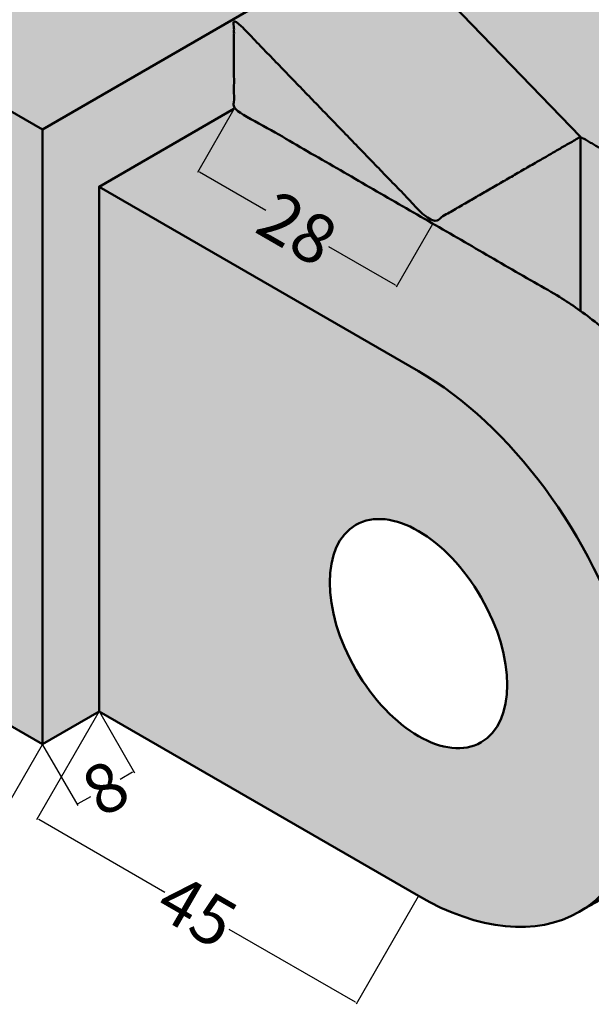
# Model space of a CAD drawing. Units: millimetres. Extents: x -24 to 183, y 0 to 191.
# Tile 1 of 1: x 51 to 120.7, y -0.5 to 119.6. Entities that reach past the tile are written whole.
import ezdxf

# ---------------------------------------------------------------- set-up
doc = ezdxf.new("R2010")
doc.units = ezdxf.units.MM
doc.header["$MEASUREMENT"] = 0
for name, color, linetype, lineweight in [('M-DIMS', 2, 'Continuous', 25), ('M-HATC', 7, 'Continuous', 18), ('M-OUTL', 7, 'Continuous', 50)]:
    doc.layers.add(name, color=color, linetype=linetype, lineweight=lineweight)
doc.styles.get("Standard").update_dxf_attribs({"font": 'arial.ttf'})
doc.dimstyles.get("Standard").update_dxf_attribs({"dimtxt": 6, "dimasz": 0.18, "dimexe": 0.18, "dimexo": 0.0625, "dimgap": 0.09, "dimtad": 0, "dimtoh": 1, "dimdec": 0, "dimzin": 0, "dimdsep": 46, "dimtxsty": 'Standard', "dimcen": 0.09, "dimadec": 0, "dimazin": 0, "dimtfac": 1, "dimtdec": 0, "dimtofl": 0, "dimtmove": 0, "dimatfit": 3, "dimfxl": 1, "dimtolj": 1, "dimtzin": 0, "dimarcsym": 0})

# ---------------------------------------------------------------- blocks, each defined once
blk = doc.blocks.new('*D2')
at = {"layer": 'Defpoints', "color": 0, "transparency": 16777216}
for p in [(77.13283570151157, 108.711638219327), (101.3815470074758, 94.71163821932711), (96.99877424901707, 87.1204531236477)]:
    blk.add_point(p, dxfattribs=at)
at = {"layer": 'M-DIMS', "color": 0, "lineweight": -2, "transparency": 16777216}
for p, q in [((77.10158570151157, 108.6575116315905), (72.6600629430528, 100.9645685509665)), ((72.905947515734, 101.0304531236477), (81.02518969457847, 96.34280646607608)), ((101.3502970074758, 94.65751163159058), (96.90877424901707, 86.9645685509665)), ((96.84288967633589, 87.2104531236477), (88.7236474974914, 91.89809978121934))]:
    blk.add_line(p, q, dxfattribs=at)
at = {"layer": 'M-DIMS', "color": 0, "transparency": 16777216}
for points in [[(72.920947515734, 101.0564338857612), (72.890947515734, 101.0044723615341), (72.7500629430528, 101.1204531236477)], [(96.85788967633587, 87.23643388576124), (96.82788967633587, 87.18447236153418), (96.99877424901707, 87.1204531236477)]]:
    blk.add_solid(points, dxfattribs=at)
at = {"layer": 'M-DIMS', "color": 0, "transparency": 16777216, "insert": (84.87441859603494, 94.1204531236477), "char_height": 6, "attachment_point": 5, "rotation": 330}
blk.add_mtext('\\A1;28', dxfattribs=at)
blk = doc.blocks.new('*D7')
at = {"layer": 'Defpoints', "color": 0, "transparency": 16777216}
for p in [(-0.8094506390879097, 62.71163821932709), (53.75014979933173, 31.2116382193271), (48.99750972183936, 22.97982413502221)]:
    blk.add_point(p, dxfattribs=at)
at = {"layer": 'M-DIMS', "color": 0, "lineweight": -2, "transparency": 16777216}
for p, q in [((-0.8407006390879097, 62.65751163159055), (-5.652090716580296, 54.32393956234097)), ((-5.406206143899098, 54.38982413502217), (17.90392502424746, 40.93171363024729)), ((48.84162514915816, 23.06982413502221), (25.53149398101159, 36.5279346397971)), ((53.71889979933173, 31.15751163159057), (48.90750972183936, 22.82393956234101))]:
    blk.add_line(p, q, dxfattribs=at)
at = {"layer": 'M-DIMS', "color": 0, "transparency": 16777216}
for points in [[(-5.391206143899097, 54.41580489713571), (-5.421206143899098, 54.36384337290864), (-5.562090716580296, 54.47982413502217)], [(48.85662514915816, 23.09580489713574), (48.82662514915816, 23.04384337290867), (48.99750972183936, 22.97982413502221)]]:
    blk.add_solid(points, dxfattribs=at)
at = {"layer": 'M-DIMS', "color": 0, "transparency": 16777216, "insert": (21.71770950262953, 38.72982413502219), "char_height": 6, "attachment_point": 5, "rotation": 330}
blk.add_mtext('\\A1;63', dxfattribs=at)
blk = doc.blocks.new('*D8')
at = {"layer": 'Defpoints', "color": 0, "transparency": 16777216}
for p in [(60.67835302960723, 35.21163821932709), (53.75014979933173, 31.2116382193271), (64.90447024958932, 27.89178847557638)]:
    blk.add_point(p, dxfattribs=at)
at = {"layer": 'M-DIMS', "color": 0, "lineweight": -2, "transparency": 16777216}
for p, q in [((60.70960302960724, 35.15751163159056), (64.99447024958933, 27.73590390289518)), ((53.78139979933172, 31.15751163159057), (58.06626701931381, 23.73590390289518)), ((64.74858567690812, 27.80178847557637), (63.23027655528555, 26.92519229549452)), ((58.13215159199502, 23.98178847557637), (59.65046071361759, 24.85838465565823))]:
    blk.add_line(p, q, dxfattribs=at)
at = {"layer": 'M-DIMS', "color": 0, "transparency": 16777216}
for points in [[(64.73358567690812, 27.8277692376899), (64.76358567690812, 27.77580771346284), (64.90447024958932, 27.89178847557638)], [(58.11715159199501, 24.00776923768991), (58.14715159199502, 23.95580771346284), (57.97626701931381, 23.89178847557637)]]:
    blk.add_solid(points, dxfattribs=at)
at = {"layer": 'M-DIMS', "color": 0, "transparency": 16777216, "insert": (61.44036863445157, 25.89178847557637), "char_height": 6, "attachment_point": 5, "rotation": 30.000000000000025}
blk.add_mtext('\\A1;8', dxfattribs=at)
blk = doc.blocks.new('*D9')
at = {"layer": 'Defpoints', "color": 0, "transparency": 16777216}
for p in [(60.67835302960723, 35.2116382193271), (99.64949619990699, 12.7116382193271), (92.11221586893467, -0.3433142648065512)]:
    blk.add_point(p, dxfattribs=at)
at = {"layer": 'M-DIMS', "color": 0, "lineweight": -2, "transparency": 16777216}
for p, q in [((60.64710302960723, 35.15751163159057), (53.0510726986349, 22.00080116251224)), ((53.2969572713161, 22.06668573519343), (68.70298209387207, 13.1720131567487)), ((99.618246199907, 12.65751163159057), (92.02221586893467, -0.4991988374877466)), ((91.95633129625347, -0.2533142648065478), (76.55030647369747, 8.6413583136382))]:
    blk.add_line(p, q, dxfattribs=at)
at = {"layer": 'M-DIMS', "color": 0, "transparency": 16777216}
for points in [[(53.31195727131611, 22.09266649730697), (53.2819572713161, 22.0407049730799), (53.1410726986349, 22.15668573519343)], [(91.97133129625345, -0.2273335026930141), (91.94133129625345, -0.2792950269200816), (92.11221586893467, -0.3433142648065512)]]:
    blk.add_solid(points, dxfattribs=at)
at = {"layer": 'M-DIMS', "color": 0, "transparency": 16777216, "insert": (72.62664428378477, 10.90668573519344), "char_height": 6, "attachment_point": 5, "rotation": 330}
blk.add_mtext('\\A1;45', dxfattribs=at)

msp = doc.modelspace()

# ---------------------------------------------------------------- hatches: boundary and pattern name
at = {"layer": 'M-HATC'}
h = msp.add_hatch(color=256, dxfattribs=at)
h.set_gradient(color1=(244, 238, 81), color2=(244, 238, 81), tint=1)
h.paths.add_polyline_path([(64.14245464474502, 175.211638219327), (-0.8094506390879131, 137.7116382193271), (53.75014979933173, 106.2116382193271), (118.7020550831646, 143.7116382193271)])
edge = h.paths.add_edge_path()
edge.add_line((95.31936918098478, 130.2116382193271), (77.13283570151161, 119.7116382193271))
edge.add_spline(control_points=[(77.13283570151158, 119.7116382193271), (89.17924906810929, 107.2566382193724), (101.2256624347508, 94.80163821937239)], knot_values=[5.356194490192345, 5.356194490192345, 5.356194490192345, 6.356194490188707, 6.356194490192345, 6.356194490192345], weights=[1, 1, 1], degree=2, periodic=0)
edge.add_spline(control_points=[(101.2256624347947, 94.80163821932707), (110.3189291745312, 100.051638219327), (119.4121959142679, 105.301638219327)], knot_values=[6.356194490188707, 6.356194490192345, 6.356194490192345, 7.356194490192345, 7.356194490192345, 7.356194490192345], weights=[1, 1, 1], degree=2, periodic=0)
edge.add_line((119.4121959142679, 105.3016382193271), (95.31936918098478, 130.2116382193271))
edge = h.paths.add_edge_path()
edge.add_spline(control_points=[(150.7449950231889, 106.2116382193271), (134.7235250531767, 115.4616382193271), (118.7020550831646, 124.7116382193271)], knot_values=[3.356194490192345, 3.356194490192345, 3.356194490192345, 4.178416712414569, 4.178416712414569, 4.178416712414569], weights=[1, 1, 1], degree=2, periodic=0)
edge.add_spline(control_points=[(118.7020550831646, 124.7116382193271), (115.2379534680269, 126.7116382193271), (111.7738518528891, 128.7116382193271)], knot_values=[4.178416712414569, 4.178416712414569, 4.178416712414569, 4.356194490192345, 4.356194490192345, 4.356194490192345], weights=[1, 1, 1], degree=2, periodic=0)
edge.add_spline(control_points=[(111.7738518528891, 128.7116382193271), (106.960071285434, 125.9324007128871), (102.1462907179789, 123.1531632064471)], knot_values=[4.356194490192345, 4.356194490192345, 4.356194490192345, 5.356194490192345, 5.356194490192345, 5.356194490192345], weights=[1, 1, 1], degree=2, periodic=0)
edge.add_line((102.1462907179789, 123.1531632064471), (119.4121959142679, 105.301638219327))
edge.add_spline(control_points=[(119.4121959142679, 105.301638219327), (126.8513541327762, 101.006638219327), (134.2905123512845, 96.71163821932709)], knot_values=[7.356194490192345, 7.356194490192345, 7.356194490192345, 8.356194490192346, 8.356194490192346, 8.356194490192346], weights=[1, 1, 1], degree=2, periodic=0)
edge.add_spline(control_points=[(134.2905123512845, 96.71163821932709), (158.0953395036126, 82.96791485491796), (161.6862132372617, 53.72180942535438), (165.2770869709107, 24.47570399579081), (142.5556009483879, 29.39608484008592)], knot_values=[8.356194490192346, 8.356194490192346, 8.356194490192346, 9.775566349411587, 9.775566349411587, 11.19493820863083, 11.19493820863083, 11.19493820863083], weights=[1, 0.7585665602715825, 1, 0.7585665602715825, 1], degree=2, periodic=0)
edge.add_spline(control_points=[(153.8864302935499, 30.77051272237281), (162.1136716295021, 35.52051272237281), (170.3409129654543, 40.2705127223728)], knot_values=[0, 0, 0, 1, 1, 1], weights=[1, 1, 1], degree=2, periodic=0)
edge.add_spline(control_points=[(170.3409129654543, 40.2705127223728), (183.4344867248955, 47.83009105704043), (176.3482956693094, 71.67543553482938), (169.2621046137232, 95.5207800126183), (150.7449950231889, 106.2116382193271)], knot_values=[1, 1, 1, 2.178097245096171, 2.178097245096171, 3.356194490192345, 3.356194490192345, 3.356194490192345], weights=[1, 0.831469612302545, 1, 0.831469612302545, 1], degree=2, periodic=0)
edge = h.paths.add_edge_path(flags=17)
edge.add_spline(control_points=[(134.2905123512845, 96.71163821932709), (126.8513541327762, 101.006638219327), (119.4121959142679, 105.301638219327)], knot_values=[7.356194490192345, 7.356194490192345, 7.356194490192345, 8.356194490192346, 8.356194490192346, 8.356194490192346], weights=[1, 1, 1], degree=2, periodic=0)
edge.add_line((119.4121959142679, 105.301638219327), (119.4121959142679, 84.07281383496964))
edge.add_spline(control_points=[(119.4121959142679, 84.07281383496964), (123.0724490086632, 81.4513939238958), (126.4903518736498, 77.88262675949477)], knot_values=[2.966768687208849, 2.966768687208849, 2.966768687208849, 3.231438789490306, 3.231438789490306, 3.231438789490306], weights=[0.9680864183363699, 0.938243390584542, 0.9254123758008628], degree=2, periodic=0)
edge.add_ellipse((134.2905123512845, 64.71163821932709), major_axis=(7.654655446197426, -13.25825214724777), ratio=0.5773502691896262, start_angle=359.3650130620468, end_angle=540.634986937953, ccw=False)
edge.add_spline(control_points=[(141.7968427812057, 51.37100682201758), (145.5119247027769, 38.61436904653682), (142.5556009483879, 29.39608484008592)], knot_values=[1.485548755374229, 1.485548755374229, 1.485548755374229, 2.169061485720957, 2.169061485720957, 2.169061485720957], weights=[0.9974346422091759, 0.9011559533067647, 0.9183363162707197], degree=2, periodic=0)
edge.add_spline(control_points=[(142.5556009483879, 29.39608484008592), (165.2770869709107, 24.47570399579081), (161.6862132372617, 53.72180942535438), (158.0953395036126, 82.96791485491796), (134.2905123512845, 96.71163821932709)], knot_values=[8.356194490192342, 8.356194490192342, 8.356194490192342, 9.775566349411587, 9.775566349411587, 11.19493820863083, 11.19493820863083, 11.19493820863083], weights=[1, 0.7585665602715825, 1, 0.7585665602715825, 1], degree=2, periodic=0)
edge = h.paths.add_edge_path()
edge.add_spline(control_points=[(119.4121959142679, 105.301638219327), (110.3189291745312, 100.051638219327), (101.2256624347947, 94.80163821932707)], knot_values=[6.356194490188707, 6.356194490188707, 6.356194490188707, 7.356194490188707, 7.356194490188707, 7.356194490192345], weights=[1, 1, 1], degree=2, periodic=0)
edge.add_spline(control_points=[(101.2256624347947, 94.80163821932709), (108.664820653303, 90.5066382193271), (116.1039788718113, 86.21163821932711)], knot_values=[3.356194490192346, 3.356194490192346, 3.356194490192346, 3.737972267970123, 3.737972267970123, 3.737972267970123], weights=[1, 1, 1], degree=2, periodic=0)
edge.add_spline(control_points=[(116.1039788718113, 86.21163821932711), (117.7640226821475, 85.25321147856292), (119.4121959142679, 84.07281383496964)], knot_values=[3.231438789490306, 3.231438789490306, 3.231438789490306, 3.356194490192346, 3.356194490192346, 3.356194490192346], weights=[1, 0.9821533182474542, 0.9680864183363699], degree=2, periodic=0)
edge.add_line((119.4121959142679, 84.07281383496965), (119.4121959142679, 105.301638219327))
h.paths.add_polyline_path([(-0.8094506390879131, 137.7116382193271), (-0.8094506390879131, 117.7116382193271), (32.09951470472076, 98.71163821932709), (32.09951470472076, 63.71163821932707), (-0.8094506390879131, 82.71163821932709), (-0.8094506390879062, 62.71163821932709), (53.75014979933173, 31.21163821932709), (53.75014979933173, 106.2116382193271)])
h.paths.add_polyline_path([(32.09951470472076, 98.71163821932709), (29.50143849336745, 100.2116382193271), (-0.8094506390879203, 82.71163821932709), (32.09951470472076, 63.71163821932708)])
edge = h.paths.add_edge_path()
edge.add_spline(control_points=[(99.64949619990696, 57.21163821932711), (99.64949619990696, 66.96163821932711), (99.64949619990696, 76.71163821932711)], knot_values=[5.141592653589794, 5.141592653589794, 5.141592653589794, 5.446280153589794, 5.446280153589794, 5.446280153589794], weights=[1, 1, 1], degree=2, periodic=0)
edge.add_line((99.64949619990699, 76.7116382193271), (60.67835302960723, 99.2116382193271))
edge.add_spline(control_points=[(60.67835302960723, 99.2116382193271), (60.67835302960723, 67.2116382193271), (60.67835302960723, 35.2116382193271)], knot_values=[0, 0, 0, 1, 1, 1], weights=[1, 1, 1], degree=2, periodic=0)
edge.add_spline(control_points=[(60.67835302960723, 35.2116382193271), (80.16392461475712, 23.9616382193271), (99.64949619990699, 12.71163821932711)], knot_values=[1, 1, 1, 2, 2, 2], weights=[1, 1, 1], degree=2, periodic=0)
edge.add_spline(control_points=[(99.64949619990699, 12.7116382193271), (99.64949619990699, 22.4616382193271), (99.64949619990699, 32.2116382193271)], knot_values=[5.836905153589794, 5.836905153589794, 5.836905153589794, 6.141592653589794, 6.141592653589794, 6.141592653589794], weights=[1, 1, 1], degree=2, periodic=0)
edge.add_ellipse((99.64949619990699, 44.7116382193271), major_axis=(7.654655446197426, -13.25825214724777), ratio=0.5773502691896261, start_angle=150, end_angle=330, ccw=False)
edge = h.paths.add_edge_path(flags=17)
edge.add_spline(control_points=[(77.13283570151158, 119.7116382193271), (77.13283570151158, 114.2116382193271), (77.13283570151158, 108.711638219327)], knot_values=[4.356194490192345, 4.356194490192345, 4.356194490192345, 5.356194490192345, 5.356194490192345, 5.356194490192345], weights=[1, 1, 1], degree=2, periodic=0)
edge.add_spline(control_points=[(77.13283570151158, 108.711638219327), (89.17924906815313, 101.7566382193271), (101.2256624347947, 94.80163821932709)], knot_values=[3.737972267970123, 3.737972267970123, 3.737972267970123, 4.356194490192345, 4.356194490192345, 4.356194490192345], weights=[1, 1, 1], degree=2, periodic=0)
edge.add_spline(control_points=[(101.2256624347508, 94.80163821937239), (89.17924906810929, 107.2566382193724), (77.13283570151158, 119.7116382193271)], knot_values=[5.356194490192345, 5.356194490192345, 5.356194490195983, 6.356194490192345, 6.356194490192345, 6.356194490192345], weights=[1, 1, 1], degree=2, periodic=0)
edge = h.paths.add_edge_path()
edge.add_spline(control_points=[(119.2454141421726, 10.77051272237291), (121.8252656817894, 12.25999070323999), (123.649496199907, 14.85523175877608), (131.649496199907, 26.23642960525908), (123.649496199907, 46.8552317587761), (115.649496199907, 67.4740339122931), (99.64949619990696, 76.71163821932711)], knot_values=[2.780860556892677, 2.780860556892677, 2.780860556892677, 3.047197551196599, 3.047197551196599, 4.094395102393195, 4.094395102393195, 5.141592653589794, 5.141592653589794, 5.141592653589794], weights=[0.9491840326991366, 0.9659258262890693, 1, 0.8660254037844385, 1, 0.8660254037844385, 1], degree=2, periodic=0)
edge.add_spline(control_points=[(99.64949619990696, 76.71163821932711), (99.64949619990696, 66.96163821932711), (99.64949619990696, 57.21163821932711)], knot_values=[5.141592653589794, 5.141592653589794, 5.141592653589794, 5.446280153589794, 5.446280153589794, 5.446280153589794], weights=[1, 1, 1], degree=2, periodic=0)
edge.add_ellipse((99.64949619990699, 44.7116382193271), major_axis=(7.654655446197426, -13.25825214724777), ratio=0.5773502691896261, start_angle=330, end_angle=509.9999999999999, ccw=False)
edge.add_spline(control_points=[(99.64949619990699, 32.2116382193271), (99.64949619990699, 22.4616382193271), (99.64949619990699, 12.7116382193271)], knot_values=[5.836905153589794, 5.836905153589794, 5.836905153589794, 6.141592653589794, 6.141592653589794, 6.141592653589794], weights=[1, 1, 1], degree=2, periodic=0)
edge.add_spline(control_points=[(99.64949619990699, 12.71163821932711), (111.1285191633359, 6.084221221357497), (119.2454141421726, 10.77051272237291)], knot_values=[2, 2, 2, 2.780860556892677, 2.780860556892677, 2.780860556892677], weights=[1, 0.9000995774953693, 0.9491840326991366], degree=2, periodic=0)
edge = h.paths.add_edge_path()
edge.add_line((118.7020550831646, 143.7116382193271), (95.31936918098478, 130.2116382193271))
edge.add_line((95.31936918098478, 130.2116382193271), (102.1462907179789, 123.1531632064471))
edge.add_spline(control_points=[(102.1462907179789, 123.1531632064471), (106.960071285434, 125.9324007128871), (111.7738518528891, 128.7116382193271)], knot_values=[4.356194490192345, 4.356194490192345, 4.356194490192345, 5.356194490192345, 5.356194490192345, 5.356194490192345], weights=[1, 1, 1], degree=2, periodic=0)
edge.add_spline(control_points=[(111.7738518528891, 128.7116382193271), (115.2379534680269, 126.7116382193271), (118.7020550831646, 124.7116382193271)], knot_values=[4.178416712414568, 4.178416712414568, 4.178416712414568, 4.356194490192344, 4.356194490192344, 4.356194490192344], weights=[1, 1, 1], degree=2, periodic=0)
edge.add_line((118.7020550831646, 124.7116382193271), (118.7020550831646, 143.7116382193271))
h = msp.add_hatch(color=256, dxfattribs=at)
h.set_gradient(color1=(244, 238, 81), color2=(244, 238, 81), tint=1)
edge = h.paths.add_edge_path()
edge.add_spline(control_points=[(77.13283570151158, 108.711638219327), (77.13283570151158, 114.2116382193271), (77.13283570151158, 119.7116382193271)], knot_values=[4.356194490192345, 4.356194490192345, 4.356194490192345, 5.356194490192345, 5.356194490192345, 5.356194490192345], weights=[1, 1, 1], degree=2, periodic=0)
edge.add_line((77.13283570151158, 119.7116382193271), (53.75014979933173, 106.2116382193271))
edge.add_line((53.75014979933173, 106.2116382193271), (53.75014979933173, 31.21163821932707))
edge.add_line((53.75014979933173, 31.21163821932707), (60.67835302960723, 35.21163821932709))
edge.add_spline(control_points=[(60.67835302960723, 35.2116382193271), (60.67835302960723, 67.2116382193271), (60.67835302960723, 99.2116382193271)], knot_values=[0, 0, 0, 1, 1, 1], weights=[1, 1, 1], degree=2, periodic=0)
edge.add_line((60.67835302960723, 99.2116382193271), (77.13283570151158, 108.7116382193271))
edge = h.paths.add_edge_path()
edge.add_spline(control_points=[(129.6626567046299, 74.29200746748931), (128.2121653973336, 76.06903189246286), (126.674769139423, 77.68917768712181)], knot_values=[2.842732393323176, 2.842732393323176, 2.842732393323176, 2.959718296587445, 2.959718296587445, 2.959718296587445], weights=[0.9171223116143046, 0.9192697655211874, 0.9247408519506481], degree=2, periodic=0)
edge.add_spline(control_points=[(126.674769139423, 77.68917768712181), (126.5826958679184, 77.78620675354577), (126.4903518736499, 77.88262675949478)], knot_values=[2.959718296587445, 2.959718296587445, 2.959718296587445, 2.966768687208849, 2.966768687208849, 2.966768687208849], weights=[0.9247408519506481, 0.925070577972116, 0.9254123758008624], degree=2, periodic=0)
edge.add_spline(control_points=[(126.4903518736499, 77.88262675949478), (125.1497541063207, 79.2823977540787), (123.7600353652503, 80.54602783327896)], knot_values=[2.966768687208849, 2.966768687208849, 2.966768687208849, 3.069712263544142, 3.069712263544142, 3.069712263544142], weights=[0.9254123758008624, 0.9304030057906388, 0.9379672558727182], degree=2, periodic=0)
edge.add_spline(control_points=[(123.7600353652503, 80.54602783327896), (122.2074968153256, 81.95770514094174), (120.6136211690738, 83.18146756875178)], knot_values=[3.069712263544142, 3.069712263544142, 3.069712263544142, 3.18671441540082, 3.18671441540082, 3.18671441540082], weights=[0.9379672558727182, 0.946564524087908, 0.9584863481523173], degree=2, periodic=0)
edge.add_spline(control_points=[(120.6136211690738, 83.18146756875178), (120.0147834077447, 83.6412494559974), (119.4121959142679, 84.07281383496966)], knot_values=[3.18671441540082, 3.18671441540082, 3.18671441540082, 3.231438789490306, 3.231438789490306, 3.231438789490306], weights=[0.9584863481523173, 0.9630434961263034, 0.9680864183363697], degree=2, periodic=0)
edge.add_spline(control_points=[(119.4121959142679, 84.07281383496966), (119.0199233503353, 84.35375372714144), (118.6264656481512, 84.62244284625048)], knot_values=[3.231438789490306, 3.231438789490306, 3.231438789490306, 3.260806039297188, 3.260806039297188, 3.260806039297188], weights=[0.9680864183363697, 0.9713977392729884, 0.9749185064116943], degree=2, periodic=0)
edge.add_spline(control_points=[(118.6264656481512, 84.62244284625048), (117.3678455130209, 85.48194447380494), (116.1039788718113, 86.21163821932711)], knot_values=[3.260806039297188, 3.260806039297188, 3.260806039297188, 3.356194490192345, 3.356194490192345, 3.356194490192345], weights=[0.9749185064116943, 0.9863543924933733, 1], degree=2, periodic=0)
edge.add_spline(control_points=[(116.1039788718113, 86.21163821932711), (111.8084928690405, 88.6916382193271), (107.5130068662697, 91.1716382193271)], knot_values=[3.356194490192345, 3.356194490192345, 3.356194490192345, 3.57663893463679, 3.57663893463679, 3.57663893463679], weights=[1, 1, 1], degree=2, periodic=0)
edge.add_spline(control_points=[(107.5130068662697, 91.1716382193271), (104.3693346505321, 92.98663821932709), (101.2256624347947, 94.80163821932709)], knot_values=[3.57663893463679, 3.57663893463679, 3.57663893463679, 3.737972267970123, 3.737972267970123, 3.737972267970123], weights=[1, 1, 1], degree=2, periodic=0)
edge.add_spline(control_points=[(101.2256624347947, 94.80163821932709), (89.18162767796578, 101.7552649283114), (77.13759292113684, 108.7088916372958)], knot_values=[3.737972267970123, 3.737972267970123, 3.737972267970123, 4.356072419879845, 4.356072419879845, 4.356072419879845], weights=[1, 1, 1], degree=2, periodic=0)
edge.add_line((77.13283570151157, 108.711638219327), (60.67835302960723, 99.2116382193271))
edge.add_line((60.67835302960723, 99.2116382193271), (99.8447195771881, 76.59892594990174))
edge.add_spline(control_points=[(99.97475492957814, 76.52164590242904), (100.1378798240307, 76.42525480692514), (100.3009708718766, 76.32666585249011)], knot_values=[5.117048971623415, 5.117048971623415, 5.117048971623415, 5.129320817599855, 5.129320817599855, 5.129320817599855], weights=[0.9968967702000623, 0.9953635526324084, 0.9938671322846566], degree=2, periodic=0)
edge.add_spline(control_points=[(100.3009708718766, 76.32666585249011), (100.6286285674363, 76.12859593973583), (100.9560124019527, 75.92173877705902)], knot_values=[5.092505444169316, 5.092505444169316, 5.092505444169316, 5.117048971623414, 5.117048971623414, 5.117048971623414], weights=[0.9938671322846566, 0.9908743116480199, 0.988028677917995], degree=2, periodic=0)
edge.add_spline(control_points=[(100.9560124019527, 75.92173877705902), (101.2862460391653, 75.71308096927459), (101.6160138777021, 75.49560053592234)], knot_values=[5.067890674546034, 5.067890674546034, 5.067890674546034, 5.092505444169316, 5.092505444169316, 5.092505444169316], weights=[0.988028677917995, 0.9851747842049658, 0.9824689331136189], degree=2, periodic=0)
edge.add_spline(control_points=[(101.6160138777021, 75.49560053592234), (102.1164304547191, 75.16557801307957), (102.6152306653907, 74.81560168592624)], knot_values=[5.030795417572638, 5.030795417572638, 5.030795417572638, 5.067890674546034, 5.067890674546034, 5.067890674546034], weights=[0.9824689331136189, 0.9783911276699186, 0.9746495487607924], degree=2, periodic=0)
edge.add_spline(control_points=[(102.6152306653907, 74.81560168592624), (103.6180936700229, 74.11195661222713), (104.6104560145192, 73.33052013900783)], knot_values=[4.957065639950063, 4.957065639950063, 4.957065639950063, 5.030795417572638, 5.030795417572638, 5.030795417572638], weights=[0.9746495487607924, 0.9672128626872858, 0.9611044304061584], degree=2, periodic=0)
edge.add_spline(control_points=[(104.6104560145192, 73.33052013900783), (105.6134251683119, 72.5407313258447), (106.6002754642349, 71.67572813658762)], knot_values=[4.883488068876007, 4.883488068876007, 4.883488068876007, 4.957065639950062, 4.957065639950062, 4.957065639950062], weights=[0.9611044304061584, 0.9550086082728485, 0.9502355615416473], degree=2, periodic=0)
edge.add_spline(control_points=[(106.6002754642349, 71.67572813658762), (108.106571986875, 70.35541511501445), (109.5597114832291, 68.87391790201954)], knot_values=[4.772588940897321, 4.772588940897321, 4.772588940897321, 4.883488068876008, 4.883488068876008, 4.883488068876008], weights=[0.9502355615416473, 0.9430414300615662, 0.9388523470348884], degree=2, periodic=0)
edge.add_spline(control_points=[(109.5597114832291, 68.87391790201954), (110.8516035735683, 67.55681480480848), (112.0878073272173, 66.12614290817397)], knot_values=[4.674819786984862, 4.674819786984862, 4.674819786984862, 4.772588940897322, 4.772588940897322, 4.772588940897322], weights=[0.9388523470348884, 0.9351592332056611, 0.9338017218698066], degree=2, periodic=0)
edge.add_spline(control_points=[(112.0878073272173, 66.12614290817397), (113.638943035053, 64.33099687458838), (115.0807423105997, 62.38251306400263)], knot_values=[4.55254402668912, 4.55254402668912, 4.55254402668912, 4.674819786984861, 4.674819786984861, 4.674819786984861], weights=[0.9338017218698066, 0.932103939654668, 0.9340593785643667], degree=2, periodic=0)
edge.add_spline(control_points=[(115.0807423105997, 62.38251306400263), (116.5292798236757, 60.42492302971401), (117.8446599635839, 58.34337763107811)], knot_values=[4.42917907937402, 4.42917907937402, 4.42917907937402, 4.55254402668912, 4.55254402668912, 4.55254402668912], weights=[0.9340593785643667, 0.9360322357969812, 0.9417236870938861], degree=2, periodic=0)
edge.add_spline(control_points=[(117.8446599635839, 58.34337763107811), (118.8713225058487, 56.71871824481724), (119.8054692643808, 55.03626807420435)], knot_values=[4.331844561881248, 4.331844561881248, 4.331844561881248, 4.42917907937402, 4.42917907937402, 4.42917907937402], weights=[0.9417236870938861, 0.9462142225164228, 0.9530196405744161], degree=2, periodic=0)
edge.add_spline(control_points=[(119.8054692643808, 55.03626807420435), (121.1922080878205, 52.53867446936446), (122.3511098193492, 49.95830163102931)], knot_values=[4.184741853008914, 4.184741853008914, 4.184741853008914, 4.331844561881248, 4.331844561881248, 4.331844561881248], weights=[0.9530196405744161, 0.9633047424799539, 0.9788771760901379], degree=2, periodic=0)
edge.add_spline(control_points=[(122.3511098193492, 49.95830163102931), (123.0447771856724, 48.41380447289763), (123.649496199907, 46.8552317587761), (123.7106124829862, 46.69771369013003), (123.7707926063305, 46.54011834809961)], knot_values=[4.085168284068898, 4.085168284068898, 4.085168284068898, 4.175515034684617, 4.175515034684617, 4.184741853008914, 4.184741853008914, 4.184741853008914], weights=[0.9788771760901379, 0.9884413696161741, 1, 0.9988195548605517, 0.9976599114367514], degree=2, periodic=0)
edge.add_spline(control_points=[(123.7707926063305, 46.54011834809961), (124.5776705294812, 44.42712496740803), (125.2107977955467, 42.31611465871429)], knot_values=[3.9634953926215, 3.9634953926215, 3.9634953926215, 4.085168284068899, 4.085168284068899, 4.085168284068899], weights=[0.9976599114367514, 0.9823678396236314, 0.9706930540319149], degree=2, periodic=0)
edge.add_spline(control_points=[(125.2107977955467, 42.31611465871429), (125.6736053367575, 40.77299443186174), (126.0393314773653, 39.24456708280777)], knot_values=[3.876368048263354, 3.876368048263354, 3.876368048263354, 3.9634953926215, 3.9634953926215, 3.9634953926215], weights=[0.9706930540319149, 0.9623329908127651, 0.9558277578449111], degree=2, periodic=0)
edge.add_spline(control_points=[(126.0393314773653, 39.24456708280777), (126.3548486882267, 37.92597078729458), (126.5961836872144, 36.62622374004979)], knot_values=[3.80214301191095, 3.80214301191095, 3.80214301191095, 3.876368048263354, 3.876368048263354, 3.876368048263354], weights=[0.9558277578449111, 0.9502858564237563, 0.9460901130582945], degree=2, periodic=0)
edge.add_spline(control_points=[(126.5961836872144, 36.62622374004979), (126.9174285486043, 34.89610974172617), (127.1046069641274, 33.21425510536911)], knot_values=[3.70435185738841, 3.70435185738841, 3.70435185738841, 3.802143011910949, 3.802143011910949, 3.802143011910949], weights=[0.9460901130582945, 0.9405622398775964, 0.9373710204515152], degree=2, periodic=0)
edge.add_spline(control_points=[(127.1046069641274, 33.21425510536911), (127.2465779563155, 31.9386028311868), (127.3104091259611, 30.69911679832556)], knot_values=[3.630620672153618, 3.630620672153618, 3.630620672153618, 3.70435185738841, 3.70435185738841, 3.70435185738841], weights=[0.9373710204515152, 0.9349649501706391, 0.9338871843993468], degree=2, periodic=0)
edge.add_spline(control_points=[(127.3104091259611, 30.69911679832556), (127.3955283033867, 29.04625610137234), (127.3411002741898, 27.47218361842691)], knot_values=[3.532563843898478, 3.532563843898478, 3.532563843898478, 3.630620672153617, 3.630620672153617, 3.630620672153617], weights=[0.9338871843993468, 0.9324538384847469, 0.9333698597606337], degree=2, periodic=0)
edge.add_spline(control_points=[(127.3411002741898, 27.47218361842691), (127.300188233985, 26.28899698356999), (127.180615341149, 25.15821918772291)], knot_values=[3.458730317071423, 3.458730317071423, 3.458730317071423, 3.532563843898478, 3.532563843898478, 3.532563843898478], weights=[0.9333698597606337, 0.9340595932820093, 0.9360813213430013], degree=2, periodic=0)
edge.add_spline(control_points=[(127.180615341149, 25.15821918772291), (127.044748511288, 23.87335277063611), (126.8083021586305, 22.66499248616322)], knot_values=[3.374446783935056, 3.374446783935056, 3.374446783935056, 3.458730317071423, 3.458730317071423, 3.458730317071423], weights=[0.9360813213430013, 0.9383891940851565, 0.9424327908815358], degree=2, periodic=0)
edge.add_spline(control_points=[(126.8083021586305, 22.66499248616322), (126.6325923480817, 21.76702660818197), (126.4021292816593, 20.91561921939569)], knot_values=[3.311341395677428, 3.311341395677428, 3.311341395677428, 3.374446783935056, 3.374446783935056, 3.374446783935056], weights=[0.9424327908815358, 0.9454603424838158, 0.9494609282808749], degree=2, periodic=0)
edge.add_spline(control_points=[(126.4021292816593, 20.91561921939569), (126.2248036377586, 20.26051918197064), (126.0155393341565, 19.63480491824097)], knot_values=[3.262421368203812, 3.262421368203812, 3.262421368203812, 3.311341395677428, 3.311341395677428, 3.311341395677428], weights=[0.9494609282808749, 0.9525622287007962, 0.9562482769267935], degree=2, periodic=0)
edge.add_spline(control_points=[(126.0155393341565, 19.63480491824097), (125.7802944825154, 18.93140707825095), (125.5053695818401, 18.26715694529732)], knot_values=[3.206973826924972, 3.206973826924972, 3.206973826924972, 3.262421368203813, 3.262421368203813, 3.262421368203813], weights=[0.9562482769267935, 0.9604261631979532, 0.9653552567738074], degree=2, periodic=0)
edge.add_spline(control_points=[(125.5053695818401, 18.26715694529732), (125.2647817315435, 17.68586906939387), (124.9944008162674, 17.13601478791239)], knot_values=[3.157982411241067, 3.157982411241067, 3.157982411241067, 3.206973826924972, 3.206973826924972, 3.206973826924972], weights=[0.9653552567738074, 0.9697104232383605, 0.9746520453803764], degree=2, periodic=0)
edge.add_spline(control_points=[(124.9944008162674, 17.13601478791239), (124.7917726002789, 16.72394431320289), (124.5727165965067, 16.33016080220038)], knot_values=[3.120938813188745, 3.120938813188745, 3.120938813188745, 3.157982411241067, 3.157982411241067, 3.157982411241067], weights=[0.9746520453803764, 0.9783885257780115, 0.9824602969029337], degree=2, periodic=0)
edge.add_spline(control_points=[(124.5727165965067, 16.33016080220038), (124.3091183628697, 15.85630646290719), (124.0221924242566, 15.40974891923198)], knot_values=[3.075952071171273, 3.075952071171273, 3.075952071171273, 3.120938813188746, 3.120938813188746, 3.120938813188746], weights=[0.9824602969029337, 0.987405165295371, 0.9928445314164283], degree=2, periodic=0)
edge.add_spline(control_points=[(124.0221924242566, 15.40974891923198), (123.8404369956832, 15.12687363048792), (123.649496199907, 14.85523175877608), (123.5683140978384, 14.73973806312165), (123.4854899919731, 14.62630190952734)], knot_values=[3.034946113864857, 3.034946113864857, 3.034946113864857, 3.063700633839531, 3.063700633839531, 3.075952071171272, 3.075952071171272, 3.075952071171272], weights=[0.9928445314164283, 0.9963212526628074, 1, 0.998432596249194, 0.9969018674291203], degree=2, periodic=0)
edge.add_spline(control_points=[(123.4854899919731, 14.62630190952734), (123.2328877991915, 14.28033715881531), (122.9652307127422, 13.95379879127234)], knot_values=[2.997811825835947, 2.997811825835947, 2.997811825835947, 3.034946113864858, 3.034946113864858, 3.034946113864858], weights=[0.9969018674291203, 0.992262205701308, 0.9879594784250201], degree=2, periodic=0)
edge.add_spline(control_points=[(122.9652307127422, 13.95379879127234), (122.6092507510389, 13.51950759758628), (122.2273513432456, 13.1204294435816)], knot_values=[2.948919902028313, 2.948919902028313, 2.948919902028313, 2.997811825835947, 2.997811825835947, 2.997811825835947], weights=[0.9879594784250201, 0.9822944010713484, 0.9772133998627793], degree=2, periodic=0)
edge.add_spline(control_points=[(122.2273513432456, 13.1204294435816), (121.9363818855874, 12.81637148574149), (121.6308038631775, 12.53322017569058)], knot_values=[2.912007262502068, 2.912007262502068, 2.912007262502068, 2.948919902028313, 2.948919902028313, 2.948919902028313], weights=[0.9772133998627793, 0.9733773232382992, 0.9698741708558454], degree=2, periodic=0)
edge.add_spline(control_points=[(121.6308038631775, 12.53322017569058), (121.2205195242283, 12.15304706261559), (120.7847527856912, 11.81133624302551)], knot_values=[2.862862349391971, 2.862862349391971, 2.862862349391971, 2.912007262502068, 2.912007262502068, 2.912007262502068], weights=[0.9698741708558454, 0.9652101283582961, 0.9611362222017703], degree=2, periodic=0)
edge.add_spline(control_points=[(120.7847527856912, 11.81133624302551), (120.4564077324761, 11.55386120576316), (120.1141041105082, 11.31863046503682)], knot_values=[2.826105434023206, 2.826105434023206, 2.826105434023206, 2.862862349391971, 2.862862349391971, 2.862862349391971], weights=[0.9611362222017703, 0.9580892288439788, 0.9553723566239481], degree=2, periodic=0)
edge.add_spline(control_points=[(120.1141041105082, 11.31863046503682), (119.7699713416554, 11.08214273621856), (119.4121959142679, 10.86845743728019)], knot_values=[2.789361644115605, 2.789361644115605, 2.789361644115605, 2.826105434023205, 2.826105434023205, 2.826105434023205], weights=[0.9553723566239481, 0.9526564545669589, 0.9502704379250916], degree=2, periodic=0)
edge.add_spline(control_points=[(119.4121959142679, 10.86680422338807), (123.4424256961962, 13.19365847288044), (127.4726554781246, 15.52051272237282)], knot_values=[0.0101359474752899, 0.0101359474752899, 0.0101359474752899, 0.5, 0.5, 0.5], weights=[1, 1, 1], degree=2, periodic=0)
edge.add_spline(control_points=[(127.4726554781246, 15.52051272237282), (131.5862761461006, 17.89551272237281), (135.6998968140767, 20.27051272237281)], knot_values=[0.5, 0.5, 0.5, 1, 1, 1], weights=[1, 1, 1], degree=2, periodic=0)
edge.add_spline(control_points=[(135.6998968140767, 20.27051272237281), (136.1539621123821, 20.53266744457909), (136.5865086976751, 20.83096823723133)], knot_values=[1, 1, 1, 1.048792481471118, 1.048792481471118, 1.048792481471118], weights=[1, 0.9930200873881364, 0.9866183397082462], degree=2, periodic=0)
edge.add_spline(control_points=[(136.5865086976751, 20.83096823723133), (136.9176670820245, 21.05934781969398), (137.2357290184705, 21.30858758031019)], knot_values=[1.048792481471118, 1.048792481471118, 1.048792481471118, 1.085724978803377, 1.085724978803377, 1.085724978803377], weights=[0.9866183397082462, 0.9817726642684901, 0.9772582444714648], degree=2, periodic=0)
edge.add_spline(control_points=[(137.2357290184705, 21.30858758031019), (137.7660086555937, 21.72412541955322), (138.2584225013502, 22.19645227598328)], knot_values=[1.085724978803377, 1.085724978803377, 1.085724978803377, 1.146550188018983, 1.146550188018983, 1.146550188018983], weights=[0.9772582444714648, 0.9698233145729854, 0.9632868744875692], degree=2, periodic=0)
edge.add_spline(control_points=[(138.2584225013502, 22.19645227598328), (138.5573675401466, 22.4832024793678), (138.8418384740707, 22.79040575169065)], knot_values=[1.146550188018983, 1.146550188018983, 1.146550188018983, 1.183078897280162, 1.183078897280162, 1.183078897280162], weights=[0.9632868744875692, 0.9593614014384435, 0.9557599803012227], degree=2, periodic=0)
edge.add_spline(control_points=[(138.8418384740707, 22.79040575169065), (139.1385886179396, 23.11086947710986), (139.4191808804897, 23.4531491801297)], knot_values=[1.183078897280162, 1.183078897280162, 1.183078897280162, 1.220893242354295, 1.220893242354295, 1.220893242354295], weights=[0.9557599803012227, 0.9520318063691403, 0.9486508959071877], degree=2, periodic=0)
edge.add_spline(control_points=[(139.4191808804897, 23.4531491801297), (139.8668572680979, 23.99924599551215), (140.2721260020161, 24.59926038119931)], knot_values=[1.220893242354295, 1.220893242354295, 1.220893242354295, 1.280671920731201, 1.280671920731201, 1.280671920731201], weights=[0.9486508959071877, 0.9433061951400592, 0.9388293321538448], degree=2, periodic=0)
edge.add_spline(control_points=[(140.2721260020161, 24.59926038119931), (140.5232608792327, 24.97107425793451), (140.7576523147468, 25.36293735961763)], knot_values=[1.280671920731201, 1.280671920731201, 1.280671920731201, 1.317431357422621, 1.317431357422621, 1.317431357422621], weights=[0.9388293321538448, 0.9360763947188564, 0.93365161576264], degree=2, periodic=0)
edge.add_spline(control_points=[(140.7576523147468, 25.36293735961763), (141.0830933170729, 25.90702004039749), (141.3755268808085, 26.48850448529568)], knot_values=[1.317431357422621, 1.317431357422621, 1.317431357422621, 1.368155388312501, 1.368155388312501, 1.368155388312501], weights=[0.93365161576264, 0.930305684112252, 0.9275845991199414], degree=2, periodic=0)
edge.add_spline(control_points=[(141.3755268808085, 26.48850448529568), (141.6466700533705, 27.02765442133951), (141.8887940808721, 27.59768818100019)], knot_values=[1.368155388312501, 1.368155388312501, 1.368155388312501, 1.414922102988684, 1.414922102988684, 1.414922102988684], weights=[0.9275845991199414, 0.9250758039155279, 0.9230981617358409], degree=2, periodic=0)
edge.add_spline(control_points=[(141.8887940808721, 27.59768818100019), (142.1766643775072, 28.2754226015726), (142.4226727061001, 28.99479987589269)], knot_values=[1.414922102988684, 1.414922102988684, 1.414922102988684, 1.470265260532734, 1.470265260532734, 1.470265260532734], weights=[0.9230981617358409, 0.9207578441943155, 0.9191613568443742], degree=2, periodic=0)
edge.add_spline(control_points=[(142.4226727061001, 28.99479987589269), (142.490760707178, 29.19390273110689), (142.5556009483879, 29.39608484008591)], knot_values=[1.470265260532734, 1.470265260532734, 1.470265260532734, 1.485548755374229, 1.485548755374229, 1.485548755374229], weights=[0.9191613568443742, 0.9187204729617025, 0.9183363162707195], degree=2, periodic=0)
edge.add_spline(control_points=[(142.5556009483879, 29.39608484008591), (142.7432960737653, 29.98134787405721), (142.9035286953098, 30.5915899432056)], knot_values=[1.485548755374229, 1.485548755374229, 1.485548755374229, 1.529718415129709, 1.529718415129709, 1.529718415129709], weights=[0.9183363162707195, 0.9172260943934935, 0.9165896714100165], degree=2, periodic=0)
edge.add_spline(control_points=[(142.9035286953098, 30.5915899432056), (143.3840015652817, 32.42145926391575), (143.6126416122373, 34.45248245982711)], knot_values=[1.529718415129709, 1.529718415129709, 1.529718415129709, 1.66179866791104, 1.66179866791104, 1.66179866791104], weights=[0.9165896714100165, 0.9146865798082515, 0.9170201297212321], degree=2, periodic=0)
edge.add_spline(control_points=[(143.6126416122373, 34.45248245982711), (143.713072375763, 35.34461493189241), (143.764143780702, 36.27047774601957)], knot_values=[1.66179866791104, 1.66179866791104, 1.66179866791104, 1.720028544551231, 1.720028544551231, 1.720028544551231], weights=[0.9170201297212321, 0.9180489157865613, 0.9199011526878917], degree=2, periodic=0)
edge.add_spline(control_points=[(143.764143780702, 36.27047774601957), (143.8286054170071, 37.43908926285298), (143.8141447210366, 38.65544637076558)], knot_values=[1.720028544551231, 1.720028544551231, 1.720028544551231, 1.793861813952505, 1.793861813952505, 1.793861813952505], weights=[0.9199011526878917, 0.9222497186478706, 0.9259221692199169], degree=2, periodic=0)
edge.add_spline(control_points=[(143.8141447210366, 38.65544637076558), (143.8028189982979, 39.60810614478695), (143.7430996364778, 40.58628027454679)], knot_values=[1.793861813952505, 1.793861813952505, 1.793861813952505, 1.852100472733457, 1.852100472733457, 1.852100472733457], weights=[0.9259221692199169, 0.9288189472915059, 0.932539424601013], degree=2, periodic=0)
edge.add_spline(control_points=[(143.7430996364778, 40.58628027454679), (143.6681967845851, 41.81315259423612), (143.517572054451, 43.07408489058984)], knot_values=[1.852100472733457, 1.852100472733457, 1.852100472733457, 1.925809061489029, 1.925809061489029, 1.925809061489029], weights=[0.932539424601013, 0.9372481719815517, 0.9432763365187515], degree=2, periodic=0)
edge.add_spline(control_points=[(143.517572054451, 43.07408489058984), (143.3419048088425, 44.54465684249924), (143.0645134371127, 46.05133158854439)], knot_values=[1.925809061489029, 1.925809061489029, 1.925809061489029, 2.012979034199378, 2.012979034199378, 2.012979034199378], weights=[0.9432763365187515, 0.9504054234687641, 0.9593798646914953], degree=2, periodic=0)
edge.add_spline(control_points=[(143.0645134371127, 46.05133158854439), (142.8323158915082, 47.31253223755684), (142.5301351100322, 48.59179692702449)], knot_values=[2.012979034199378, 2.012979034199378, 2.012979034199378, 2.08722275193102, 2.08722275193102, 2.08722275193102], weights=[0.9593798646914953, 0.9670235045851738, 0.9760057892826022], degree=2, periodic=0)
edge.add_spline(control_points=[(142.5301351100322, 48.59179692702449), (142.2034215698478, 49.97491961764523), (141.7968427812057, 51.37100682201758)], knot_values=[2.08722275193102, 2.08722275193102, 2.08722275193102, 2.169061485720957, 2.169061485720957, 2.169061485720957], weights=[0.9760057892826022, 0.9859069476383204, 0.9974346422091759], degree=2, periodic=0)
edge.add_spline(control_points=[(141.7968427812057, 51.37100682201758), (141.7525280489804, 51.52317223829919), (141.7072795179318, 51.67543553482938), (141.6624929613182, 51.82614426707313), (141.6167947871972, 51.97693808478169)], knot_values=[2.169061485720957, 2.169061485720957, 2.169061485720957, 2.178097245096171, 2.178097245096171, 2.187040870006556, 2.187040870006556, 2.187040870006556], weights=[0.9974346422091759, 0.9987074071881719, 1, 0.9987205873030927, 0.9974606001456546], degree=2, periodic=0)
edge.add_spline(control_points=[(141.6167947871972, 51.97693808478169), (140.9517794604651, 54.17134085647821), (140.0997815197228, 56.36604687055694)], knot_values=[2.187040870006556, 2.187040870006556, 2.187040870006556, 2.314683904073241, 2.314683904073241, 2.314683904073241], weights=[0.9974606001456546, 0.9794781170616754, 0.965452398201826], degree=2, periodic=0)
edge.add_spline(control_points=[(140.0997815197228, 56.36604687055694), (139.2839372106333, 58.46762285576458), (138.3081005691592, 60.53982325286182)], knot_values=[2.314683904073241, 2.314683904073241, 2.314683904073241, 2.433530685609216, 2.433530685609216, 2.433530685609216], weights=[0.965452398201826, 0.9523932324008108, 0.9427642772030161], degree=2, periodic=0)
edge.add_spline(control_points=[(138.3081005691592, 60.53982325286182), (137.0861762910274, 63.13459359325666), (135.6376199164575, 65.63298565436963)], knot_values=[2.433530685609216, 2.433530685609216, 2.433530685609216, 2.579002148155839, 2.579002148155839, 2.579002148155839], weights=[0.9427642772030161, 0.9309781928234816, 0.9243313797502773], degree=2, periodic=0)
edge.add_spline(control_points=[(135.6376199164575, 65.63298565436963), (134.4574971723731, 67.66839783902462), (133.1455600512967, 69.60716400973533)], knot_values=[2.579002148155839, 2.579002148155839, 2.579002148155839, 2.695989522507838, 2.695989522507838, 2.695989522507838], weights=[0.9243313797502773, 0.9189860481255712, 0.9169644326127578], degree=2, periodic=0)
edge.add_spline(control_points=[(133.1455600512967, 69.60716400973533), (131.4917327990659, 72.05117163579708), (129.6626567046299, 74.29200746748931)], knot_values=[2.695989522507838, 2.695989522507838, 2.695989522507838, 2.842732393323176, 2.842732393323176, 2.842732393323176], weights=[0.9169644326127578, 0.9144286233796822, 0.9171223116143046], degree=2, periodic=0)
h.paths.add_polyline_path([(76.47887617717802, 91.77949279967994), (87.15119196487902, 85.61782840677407), (93.33332020498817, 96.32558861754949), (82.66100441728715, 102.4872530104553)], flags=24)

# ---------------------------------------------------------------- linework, layer by layer
at = {"layer": 'M-OUTL'}
for p, q in [((60.67832972377784, 35.21155000000001), (60.67832972377784, 99.21155000000002)), ((99.64947289407758, 12.71154999999999), (60.67832972377784, 35.21155))]:
    msp.add_line(p, q, dxfattribs=at)
for points in [[(53.75014979933173, 106.2116382193271), (-0.8094506390879131, 137.7116382193271), (64.14245464474502, 175.211638219327), (118.7020550831646, 143.7116382193271), (118.7020550831646, 124.7116382193271)], [(60.67835302960723, 35.21163821932709), (53.75014979933173, 31.2116382193271), (53.75014979933173, 106.2116382193271), (118.7020550831646, 143.7116382193271)], [(95.31936918098476, 130.2116382193271), (119.4121959142679, 105.301638219327), (119.4121959142679, 84.07281383496965)], [(77.13283570151158, 108.7116382193271), (60.67835302960723, 99.2116382193271), (99.64949619990696, 76.7116382193271)], [(53.75014979933173, 31.2116382193271), (-0.8094506390879131, 62.71163821932709), (-0.8094506390879131, 82.71163821932709)], [(119.4121959142679, 10.8684574372802), (119.4121959142679, 10.86680422338807)]]:
    msp.add_lwpolyline(points, dxfattribs=at)
for start_param, end_param in [(2e-16, 2.356194490192344), (5.497787143782137, 6.283185307179586)]:
    msp.add_ellipse((99.64947289407758, 44.71155), major_axis=(19.59591794226542, -33.94112549695428), ratio=0.5773502691896258, start_param=start_param, end_param=end_param, dxfattribs=at)
msp.add_ellipse((99.64949619990699, 44.7116382193271), major_axis=(7.654655446197422, -13.25825214724777), ratio=0.5773502691896262, dxfattribs=at)
for points, weights, knots in [([(153.8864302935499, 30.77051272237281), (162.1136716295021, 35.52051272237281), (170.3409129654543, 40.2705127223728), (183.4344867248955, 47.83009105704043), (176.3482956693094, 71.67543553482938), (169.2621046137232, 95.5207800126183), (150.7449950231889, 106.2116382193271), (131.259423438039, 117.4616382193271), (111.7738518528891, 128.7116382193271), (106.960071285434, 125.9324007128871), (102.1462907179789, 123.1531632064471)], [1, 1, 1, 0.831469612302545, 1, 0.831469612302545, 1, 1, 1, 1, 1], [0, 0, 0, 1, 1, 2.178097245096171, 2.178097245096171, 3.356194490192345, 3.356194490192345, 4.356194490192345, 4.356194490192345, 5.356194490192345, 5.356194490192345, 5.356194490192345]), ([(119.2454141421724, 10.77051272237282), (127.4726554781246, 15.52051272237282), (135.6998968140767, 20.27051272237281), (148.793470573518, 27.83009105704043), (141.7072795179318, 51.67543553482938), (134.6210884623456, 75.52078001261833), (116.1039788718113, 86.21163821932711), (96.61840728666145, 97.46163821932709), (77.13283570151158, 108.711638219327), (77.13283570151158, 114.2116382193271), (77.13283570151158, 119.7116382193271), (89.17924906815313, 107.2566382193271), (101.2256624347947, 94.80163821932707), (110.3189291745312, 100.051638219327), (119.4121959142679, 105.301638219327), (126.8513541327762, 101.006638219327), (134.2905123512845, 96.71163821932709), (158.0953395036126, 82.96791485491796), (161.6862132372617, 53.72180942535438), (165.2770869709107, 24.47570399579081), (142.5556009483879, 29.39608484008592)], [1, 1, 1, 0.831469612302545, 1, 0.831469612302545, 1, 1, 1, 1, 1, 1, 1, 1, 1, 1, 1, 0.7585665602715825, 1, 0.7585665602715825, 1], [0, 0, 0, 1, 1, 2.178097245096171, 2.178097245096171, 3.356194490192345, 3.356194490192345, 4.356194490192345, 4.356194490192345, 5.356194490192345, 5.356194490192345, 6.356194490192345, 6.356194490192345, 7.356194490192345, 7.356194490192345, 8.356194490192346, 8.356194490192346, 9.775566349411587, 9.775566349411587, 11.19493820863083, 11.19493820863083, 11.19493820863083])]:
    msp.add_rational_spline(points, weights, degree=2, knots=knots, dxfattribs=at)

# ---------------------------------------------------------------- dimensions: what is measured, and where the dimension line sits
at = {"layer": 'M-DIMS'}
for p1, p2, distance, picture, middle in [((77.13283570151158, 108.7116382193271), (101.3815470074758, 94.71163821932711), -8.765545516917534, '*D2', (84.87441859603494, 94.1204531236477)), ((-0.8094506390879131, 62.71163821932709), (53.75014979933173, 31.2116382193271), -9.505280154984762, '*D7', (21.71770950262953, 38.72982413502219)), ((60.67835302960723, 35.21163821932709), (99.64949619990699, 12.7116382193271), -15.074560661944666, '*D9', (72.62664428378477, 10.90668573519344)), ((53.75014979933173, 31.2116382193271), (60.67835302960723, 35.21163821932709), -8.452234439964178, '*D8', (61.44036863445157, 25.89178847557637))]:
    dim = msp.add_aligned_dim(p1=p1, p2=p2, distance=distance, dimstyle='Standard', override={"dimclrd": 0, "dimclre": 0, "dimclrt": 0}, dxfattribs=at)
    dim.commit()
    dim.dimension.update_dxf_attribs({"geometry": picture, "text_midpoint": middle})

doc.saveas('drawing.dxf')
